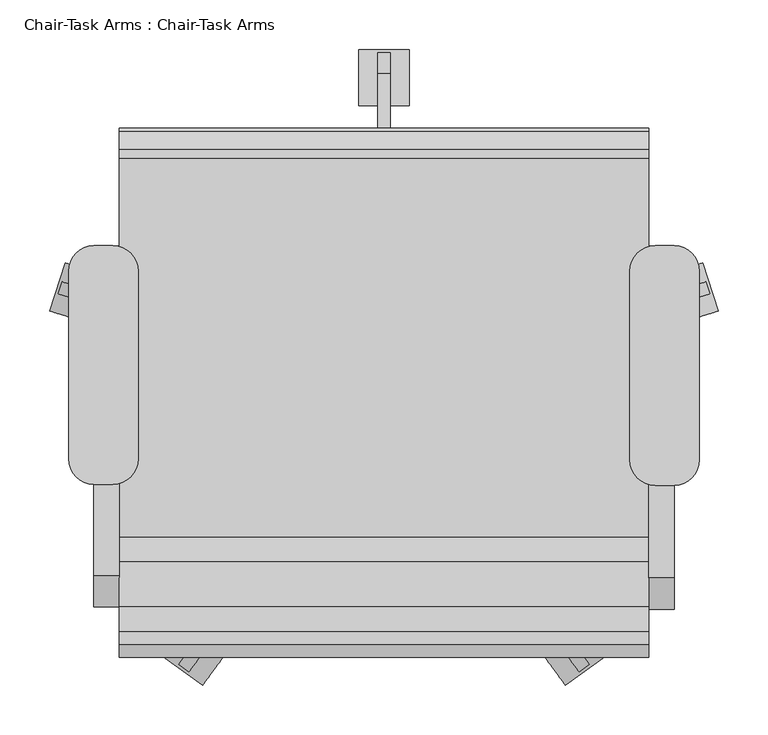
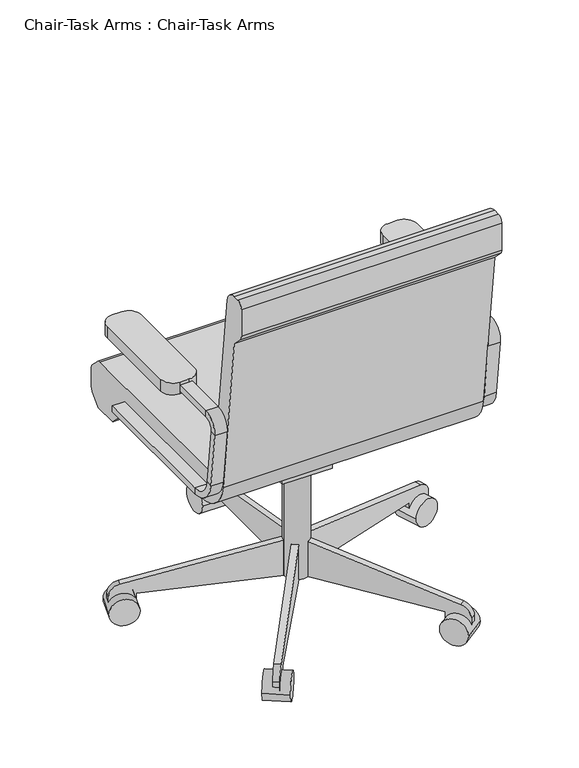
"""IFC4 building model written with IfcOpenShell, lengths in millimetres: furniture geometry, Chair-Task Arms : Chair-Task Arms."""

from ifc_helpers import new_model, si_unit, point, frame, frame_2d, origin, place, context, project, spatial, polyline, circle_curve, trimmed, segment, composite_curve, outline, extrude, source, transform, mapped, element, save
from ifc_brep_helpers import plane_surface, cylinder_surface, revolved_surface, advanced_brep


def chair_task_arms_chair_task_arms_fa5a08ef(model_context):
    return source(origin(), model_context, "Body", "SolidModel", [
        extrude(outline(composite_curve([segment(polyline([(433.0908197, -74.2028048), (414.0408197, -74.2028048)]), True, "CONTINUOUS"), segment(trimmed(circle_curve(frame_2d((414.0408197, -48.8028048)), 25.4), [point((414.0408197, -74.2028048))], [point((388.6408197, -48.8028048))], False, "CARTESIAN"), True, "CONTINUOUS"), segment(polyline([(388.6408197, -48.8028048), (388.6408197, 141.6319091)]), True, "CONTINUOUS"), segment(trimmed(circle_curve(frame_2d((414.0408197, 141.6319091)), 25.4), [point((388.6408197, 141.6319091))], [point((414.0408197, 167.0319091))], False, "CARTESIAN"), True, "CONTINUOUS"), segment(polyline([(414.0408197, 167.0319091), (433.0908197, 167.0319091)]), True, "CONTINUOUS"), segment(trimmed(circle_curve(frame_2d((433.0908197, 141.6319091)), 25.4), [point((433.0908197, 167.0319091))], [point((458.4908197, 141.6319091))], False, "CARTESIAN"), True, "CONTINUOUS"), segment(polyline([(458.4908197, 141.6319091), (458.4908197, -48.8028048)]), True, "CONTINUOUS"), segment(trimmed(circle_curve(frame_2d((433.0908197, -48.8028048)), 25.4), [point((458.4908197, -48.8028048))], [point((433.0908197, -74.2028048))], False, "CARTESIAN"), True, "CONTINUOUS")], self_intersect=False)), frame((0.0, 0.0, 596.9), z_axis=(0.0, 0.0, 1.0), x_axis=(1.0, 0.0, 0.0)), (0.0, 0.0, 1.0), 25.4),
        extrude(outline(composite_curve([segment(polyline([(-132.0591803, -73.1575984), (-151.1091803, -73.1575984)]), True, "CONTINUOUS"), segment(trimmed(circle_curve(frame_2d((-151.1091803, -47.7575984)), 25.4), [point((-151.1091803, -73.1575984))], [point((-176.5091803, -47.7575984))], False, "CARTESIAN"), True, "CONTINUOUS"), segment(polyline([(-176.5091803, -47.7575984), (-176.5091803, 141.6319091)]), True, "CONTINUOUS"), segment(trimmed(circle_curve(frame_2d((-151.1091803, 141.6319091)), 25.4), [point((-176.5091803, 141.6319091))], [point((-151.1091803, 167.0319091))], False, "CARTESIAN"), True, "CONTINUOUS"), segment(polyline([(-151.1091803, 167.0319091), (-132.0591803, 167.0319091)]), True, "CONTINUOUS"), segment(trimmed(circle_curve(frame_2d((-132.0591803, 141.6319091)), 25.4), [point((-132.0591803, 167.0319091))], [point((-106.6591803, 141.6319091))], False, "CARTESIAN"), True, "CONTINUOUS"), segment(polyline([(-106.6591803, 141.6319091), (-106.6591803, -47.7575984)]), True, "CONTINUOUS"), segment(trimmed(circle_curve(frame_2d((-132.0591803, -47.7575984)), 25.4), [point((-106.6591803, -47.7575984))], [point((-132.0591803, -73.1575984))], False, "CARTESIAN"), True, "CONTINUOUS")], self_intersect=False)), frame((0.0, 0.0, 596.9), z_axis=(0.0, 0.0, 1.0), x_axis=(1.0, 0.0, 0.0)), (0.0, 0.0, 1.0), 25.4),
        advanced_brep(
        [(-151.1091803, 167.0319091, 412.75), (-151.1091803, 167.0319091, 425.45), (-125.7091803, 167.0319091, 425.45), (-125.7091803, 167.0319091, 412.75), (-151.1091803, -126.2388651, 412.75), (-151.1091803, -126.2388651, 425.45), (-125.7091803, -126.2388651, 425.45), (-125.7091803, -126.2388651, 412.75), (-151.1091803, -170.3844094, 464.7064065), (-151.1091803, -182.9974221, 463.2225227), (-125.7091803, -170.3844094, 464.7064065), (-125.7091803, -182.9974221, 463.2225227), (-151.1091803, -196.7936301, 580.4902904), (-151.1091803, -184.1806174, 581.9741742), (-125.7091803, -184.1806174, 581.9741742), (-125.7091803, -196.7936301, 580.4902904), (-151.1091803, -165.2610984, 603.25), (-151.1091803, -165.2610984, 615.95), (-125.7091803, -165.2610984, 603.25), (-125.7091803, -165.2610984, 615.95), (-151.1091803, 18.9459016, 615.95), (-125.7091803, 18.9459016, 615.95), (-125.7091803, 18.9459016, 603.25), (-151.1091803, 18.9459016, 603.25)],
        [
            (0, 1),
            (1, 2),
            (2, 3),
            (3, 0),
            (0, 4),
            (4, 5),
            (5, 1),
            (5, 6),
            (6, 2),
            (6, 7),
            (7, 3),
            (7, 4),
            (8, 5, circle_curve(frame((-151.1091803, -126.2388651, 469.9), z_axis=(1.0, 0.0, 0.0), x_axis=(0.0, 0.0, -1.0)), 44.45)),
            (4, 9, circle_curve(frame((-151.1091803, -126.2388651, 469.9), z_axis=(-1.0, 0.0, 0.0), x_axis=(0.0, 0.0, -1.0)), 57.15)),
            (9, 8),
            (10, 6, circle_curve(frame((-125.7091803, -126.2388651, 469.9), z_axis=(1.0, 0.0, 0.0), x_axis=(0.0, 0.0, -1.0)), 44.45)),
            (8, 10),
            (11, 7, circle_curve(frame((-125.7091803, -126.2388651, 469.9), z_axis=(1.0, 0.0, 0.0), x_axis=(0.0, 0.0, -1.0)), 57.15)),
            (10, 11),
            (11, 9),
            (9, 12),
            (12, 13),
            (13, 8),
            (13, 14),
            (14, 10),
            (14, 15),
            (15, 11),
            (15, 12),
            (16, 13, circle_curve(frame((-151.1091803, -165.2610984, 584.2), z_axis=(1.0, 0.0, 0.0), x_axis=(0.0, -0.9931506043228768, -0.11684124756739202)), 19.05)),
            (12, 17, circle_curve(frame((-151.1091803, -165.2610984, 584.2), z_axis=(-1.0, 0.0, 0.0), x_axis=(0.0, -0.9931506043228768, -0.11684124756739202)), 31.75)),
            (17, 16),
            (18, 14, circle_curve(frame((-125.7091803, -165.2610984, 584.2), z_axis=(1.0, 0.0, 0.0), x_axis=(0.0, -0.9931506043228768, -0.11684124756739202)), 19.05)),
            (16, 18),
            (19, 15, circle_curve(frame((-125.7091803, -165.2610984, 584.2), z_axis=(1.0, 0.0, 0.0), x_axis=(0.0, -0.9931506043228768, -0.11684124756739202)), 31.75)),
            (18, 19),
            (19, 17),
            (20, 21),
            (21, 22),
            (22, 23),
            (23, 20),
            (17, 20),
            (23, 16),
            (22, 18),
            (21, 19),
        ],
        [
            plane_surface(frame((-152.608212, 167.0319091, 419.1), z_axis=(0.0, 1.0, 0.0), x_axis=(0.0, 0.0, -1.0))),
            plane_surface(frame((-151.1091803, 167.0319091, 412.75), z_axis=(-1.0, 0.0, 0.0), x_axis=(0.0, -1.0, 0.0))),
            plane_surface(frame((-151.1091803, 167.0319091, 425.45), z_axis=(0.0, 0.0, 1.0), x_axis=(0.0, -1.0, 0.0))),
            plane_surface(frame((-125.7091803, 167.0319091, 425.45), z_axis=(1.0, 0.0, 0.0), x_axis=(0.0, -1.0, 0.0))),
            plane_surface(frame((-125.7091803, 167.0319091, 412.75), z_axis=(0.0, 0.0, -1.0), x_axis=(0.0, -1.0, 0.0))),
            plane_surface(frame((-151.1091803, -126.2388651, 469.9), z_axis=(-1.0, 0.0, 0.0), x_axis=(0.0, 0.0, -1.0))),
            revolved_surface(polyline([(-151.1091803, -126.2388651, 425.45), (-125.7091803, -126.2388651, 425.45)]), (-138.4091803, -126.2388651, 469.9), (-1.0, 0.0, 0.0)),
            plane_surface(frame((-125.7091803, -126.2388651, 469.9), z_axis=(1.0, 0.0, 0.0), x_axis=(0.0, 0.0, -1.0))),
            cylinder_surface(frame((-138.4091803, -126.2388651, 469.9), z_axis=(-1.0, 0.0, 0.0), x_axis=(0.0, 0.0, -1.0)), 57.15),
            plane_surface(frame((-151.1091803, -182.9974221, 463.2225227), z_axis=(-1.0, 0.0, 0.0), x_axis=(0.0, -0.1168412475673856, 0.9931506043228776))),
            plane_surface(frame((-151.1091803, -170.3844094, 464.7064065), z_axis=(0.0, 0.9931506043228776, 0.1168412475673856), x_axis=(0.0, -0.1168412475673856, 0.9931506043228776))),
            plane_surface(frame((-125.7091803, -170.3844094, 464.7064065), z_axis=(1.0, 0.0, 0.0), x_axis=(0.0, -0.1168412475673856, 0.9931506043228776))),
            plane_surface(frame((-125.7091803, -182.9974221, 463.2225227), z_axis=(0.0, -0.9931506043228776, -0.1168412475673856), x_axis=(0.0, -0.1168412475673856, 0.9931506043228776))),
            plane_surface(frame((-151.1091803, -165.2610984, 584.2), z_axis=(-1.0, 0.0, 0.0), x_axis=(0.0, -0.9931506043228768, -0.11684124756739202))),
            revolved_surface(polyline([(-151.1091803, -184.1806174123508, 581.9741742338413), (-125.7091803, -184.1806174123508, 581.9741742338413)]), (-138.4091803, -165.2610984, 584.2), (-1.0, 0.0, 0.0)),
            plane_surface(frame((-125.7091803, -165.2610984, 584.2), z_axis=(1.0, 0.0, 0.0), x_axis=(0.0, -0.9931506043228768, -0.11684124756739202))),
            cylinder_surface(frame((-138.4091803, -165.2610984, 584.2), z_axis=(-1.0, 0.0, 0.0), x_axis=(0.0, -0.9931506043228768, -0.11684124756739202)), 31.75),
            plane_surface(frame((-152.608212, 18.9459016, 609.6), z_axis=(0.0, 1.0, 0.0), x_axis=(0.0, 0.0, 1.0))),
            plane_surface(frame((-151.1091803, -165.2610984, 615.95), z_axis=(-1.0, 0.0, 0.0), x_axis=(0.0, 1.0, 0.0))),
            plane_surface(frame((-151.1091803, -165.2610984, 603.25), z_axis=(0.0, 0.0, -1.0), x_axis=(0.0, 1.0, 0.0))),
            plane_surface(frame((-125.7091803, -165.2610984, 603.25), z_axis=(1.0, 0.0, 0.0), x_axis=(0.0, 1.0, 0.0))),
            plane_surface(frame((-125.7091803, -165.2610984, 615.95), z_axis=(0.0, 0.0, 1.0), x_axis=(0.0, 1.0, 0.0))),
        ],
        [
            (0, [[1, 2, 3, 4]]),
            (1, [[-1, 5, 6, 7]]),
            (2, [[-2, -7, 8, 9]]),
            (3, [[-3, -9, 10, 11]]),
            (4, [[-4, -11, 12, -5]]),
            (5, [[13, -6, 14, 15]]),
            (6, [[16, -8, -13, 17]]),
            (7, [[18, -10, -16, 19]]),
            (8, [[-14, -12, -18, 20]]),
            (9, [[-15, 21, 22, 23]]),
            (10, [[-17, -23, 24, 25]]),
            (11, [[-19, -25, 26, 27]]),
            (12, [[-20, -27, 28, -21]]),
            (13, [[29, -22, 30, 31]]),
            (14, [[32, -24, -29, 33]]),
            (15, [[34, -26, -32, 35]]),
            (16, [[-30, -28, -34, 36]]),
            (17, [[37, 38, 39, 40]]),
            (18, [[-31, 41, -40, 42]]),
            (19, [[-33, -42, -39, 43]]),
            (20, [[-35, -43, -38, 44]]),
            (21, [[-36, -44, -37, -41]]),
        ],
    ),
        advanced_brep(
        [(433.0908197, 167.0319091, 425.45), (433.0908197, 167.0319091, 412.75), (407.6908197, 167.0319091, 412.75), (407.6908197, 167.0319091, 425.45), (433.0908197, -128.329278, 425.45), (433.0908197, -128.329278, 412.75), (407.6908197, -128.329278, 412.75), (407.6908197, -128.329278, 425.45), (433.0908197, -185.0878351, 463.2225227), (433.0908197, -172.4748224, 464.7064065), (407.6908197, -185.0878351, 463.2225227), (407.6908197, -172.4748224, 464.7064065), (433.0908197, -186.2710303, 581.9741742), (433.0908197, -198.884043, 580.4902904), (407.6908197, -198.884043, 580.4902904), (407.6908197, -186.2710303, 581.9741742), (433.0908197, -167.3515113, 615.95), (433.0908197, -167.3515113, 603.25), (407.6908197, -167.3515113, 615.95), (407.6908197, -167.3515113, 603.25), (433.0908197, 18.9459016, 603.25), (407.6908197, 18.9459016, 603.25), (407.6908197, 18.9459016, 615.95), (433.0908197, 18.9459016, 615.95)],
        [
            (0, 1),
            (1, 2),
            (2, 3),
            (3, 0),
            (0, 4),
            (4, 5),
            (5, 1),
            (5, 6),
            (6, 2),
            (6, 7),
            (7, 3),
            (7, 4),
            (8, 5, circle_curve(frame((433.0908197, -128.329278, 469.9), z_axis=(1.0, 0.0, 0.0), x_axis=(0.0, 0.0, -1.0)), 57.15)),
            (4, 9, circle_curve(frame((433.0908197, -128.329278, 469.9), z_axis=(-1.0, 0.0, 0.0), x_axis=(0.0, 0.0, -1.0)), 44.45)),
            (9, 8),
            (10, 6, circle_curve(frame((407.6908197, -128.329278, 469.9), z_axis=(1.0, 0.0, 0.0), x_axis=(0.0, 0.0, -1.0)), 57.15)),
            (8, 10),
            (11, 7, circle_curve(frame((407.6908197, -128.329278, 469.9), z_axis=(1.0, 0.0, 0.0), x_axis=(0.0, 0.0, -1.0)), 44.45)),
            (10, 11),
            (11, 9),
            (9, 12),
            (12, 13),
            (13, 8),
            (13, 14),
            (14, 10),
            (14, 15),
            (15, 11),
            (15, 12),
            (16, 13, circle_curve(frame((433.0908197, -167.3515113, 584.2), z_axis=(1.0, 0.0, 0.0), x_axis=(0.0, -0.9931506043228767, -0.1168412475673929)), 31.75)),
            (12, 17, circle_curve(frame((433.0908197, -167.3515113, 584.2), z_axis=(-1.0, 0.0, 0.0), x_axis=(0.0, -0.9931506043228767, -0.1168412475673929)), 19.05)),
            (17, 16),
            (18, 14, circle_curve(frame((407.6908197, -167.3515113, 584.2), z_axis=(1.0, 0.0, 0.0), x_axis=(0.0, -0.9931506043228767, -0.1168412475673929)), 31.75)),
            (16, 18),
            (19, 15, circle_curve(frame((407.6908197, -167.3515113, 584.2), z_axis=(1.0, 0.0, 0.0), x_axis=(0.0, -0.9931506043228767, -0.1168412475673929)), 19.05)),
            (18, 19),
            (19, 17),
            (20, 21),
            (21, 22),
            (22, 23),
            (23, 20),
            (17, 20),
            (23, 16),
            (22, 18),
            (21, 19),
        ],
        [
            plane_surface(frame((406.191788, 167.0319091, 419.1), z_axis=(0.0, 1.0, 0.0), x_axis=(0.0, 0.0, -1.0))),
            plane_surface(frame((433.0908197, 167.0319091, 425.45), z_axis=(1.0, 0.0, 0.0), x_axis=(0.0, -1.0, 0.0))),
            plane_surface(frame((433.0908197, 167.0319091, 412.75), z_axis=(0.0, 0.0, -1.0), x_axis=(0.0, -1.0, 0.0))),
            plane_surface(frame((407.6908197, 167.0319091, 412.75), z_axis=(-1.0, 0.0, 0.0), x_axis=(0.0, -1.0, 0.0))),
            plane_surface(frame((407.6908197, 167.0319091, 425.45), z_axis=(0.0, 0.0, 1.0), x_axis=(0.0, -1.0, 0.0))),
            plane_surface(frame((433.0908197, -128.329278, 469.9), z_axis=(1.0, 0.0, 0.0), x_axis=(0.0, 0.0, -1.0))),
            cylinder_surface(frame((420.3908197, -128.329278, 469.9), z_axis=(-1.0, 0.0, 0.0), x_axis=(0.0, 0.0, -1.0)), 57.15),
            plane_surface(frame((407.6908197, -128.329278, 469.9), z_axis=(-1.0, 0.0, 0.0), x_axis=(0.0, 0.0, -1.0))),
            revolved_surface(polyline([(407.6908197, -128.329278, 425.45), (433.0908197, -128.329278, 425.45)]), (420.3908197, -128.329278, 469.9), (-1.0, 0.0, 0.0)),
            plane_surface(frame((433.0908197, -172.4748224, 464.7064065), z_axis=(1.0, 0.0, 0.0), x_axis=(0.0, -0.11684124756738626, 0.9931506043228775))),
            plane_surface(frame((433.0908197, -185.0878351, 463.2225227), z_axis=(0.0, -0.9931506043228775, -0.11684124756738655), x_axis=(0.0, -0.11684124756738655, 0.9931506043228775))),
            plane_surface(frame((407.6908197, -185.0878351, 463.2225227), z_axis=(-1.0, 0.0, 0.0), x_axis=(0.0, -0.11684124756738626, 0.9931506043228775))),
            plane_surface(frame((407.6908197, -172.4748224, 464.7064065), z_axis=(0.0, 0.9931506043228775, 0.11684124756738626), x_axis=(0.0, -0.11684124756738626, 0.9931506043228775))),
            plane_surface(frame((433.0908197, -167.3515113, 584.2), z_axis=(1.0, 0.0, 0.0), x_axis=(0.0, -0.9931506043228767, -0.1168412475673929))),
            cylinder_surface(frame((420.3908197, -167.3515113, 584.2), z_axis=(-1.0, 0.0, 0.0), x_axis=(0.0, -0.9931506043228767, -0.1168412475673929)), 31.75),
            plane_surface(frame((407.6908197, -167.3515113, 584.2), z_axis=(-1.0, 0.0, 0.0), x_axis=(0.0, -0.9931506043228767, -0.1168412475673929))),
            revolved_surface(polyline([(407.6908197, -186.2710303123508, 581.9741742338412), (433.0908197, -186.2710303123508, 581.9741742338412)]), (420.3908197, -167.3515113, 584.2), (-1.0, 0.0, 0.0)),
            plane_surface(frame((406.191788, 18.9459016, 609.6), z_axis=(0.0, 1.0, 0.0), x_axis=(0.0, 0.0, 1.0))),
            plane_surface(frame((433.0908197, -167.3515113, 603.25), z_axis=(1.0, 0.0, 0.0), x_axis=(0.0, 1.0, 0.0))),
            plane_surface(frame((433.0908197, -167.3515113, 615.95), z_axis=(0.0, 0.0, 1.0), x_axis=(0.0, 1.0, 0.0))),
            plane_surface(frame((407.6908197, -167.3515113, 615.95), z_axis=(-1.0, 0.0, 0.0), x_axis=(0.0, 1.0, 0.0))),
            plane_surface(frame((407.6908197, -167.3515113, 603.25), z_axis=(0.0, 0.0, -1.0), x_axis=(0.0, 1.0, 0.0))),
        ],
        [
            (0, [[1, 2, 3, 4]]),
            (1, [[-1, 5, 6, 7]]),
            (2, [[-2, -7, 8, 9]]),
            (3, [[-3, -9, 10, 11]]),
            (4, [[-4, -11, 12, -5]]),
            (5, [[13, -6, 14, 15]]),
            (6, [[16, -8, -13, 17]]),
            (7, [[18, -10, -16, 19]]),
            (8, [[-14, -12, -18, 20]]),
            (9, [[-15, 21, 22, 23]]),
            (10, [[-17, -23, 24, 25]]),
            (11, [[-19, -25, 26, 27]]),
            (12, [[-20, -27, 28, -21]]),
            (13, [[29, -22, 30, 31]]),
            (14, [[32, -24, -29, 33]]),
            (15, [[34, -26, -32, 35]]),
            (16, [[-30, -28, -34, 36]]),
            (17, [[37, 38, 39, 40]]),
            (18, [[-31, 41, -40, 42]]),
            (19, [[-33, -42, -39, 43]]),
            (20, [[-35, -43, -38, 44]]),
            (21, [[-36, -44, -37, -41]]),
        ],
    ),
        extrude(outline(composite_curve([segment(trimmed(circle_curve(frame_2d((140.9908197, 18.9459016)), 25.4), [point((115.5908197, 18.9459016))], [point((166.3908197, 18.9459016))], False, "CARTESIAN"), True, "CONTINUOUS"), segment(trimmed(circle_curve(frame_2d((140.9908197, 18.9459016)), 25.4), [point((166.3908197, 18.9459016))], [point((115.5908197, 18.9459016))], False, "CARTESIAN"), True, "CONTINUOUS")], self_intersect=False)), frame((0.0, 0.0, 53.5835944), z_axis=(0.0, 0.0, 1.0), x_axis=(1.0, 0.0, 0.0)), (0.0, 0.0, 1.0), 330.5914056),
        extrude(outline(composite_curve([segment(trimmed(circle_curve(frame_2d((0.0, -28.2002727)), 28.2002727), [point((0.0, -56.4005455))], [point((0.0, 0.0))], False, "CARTESIAN"), True, "CONTINUOUS"), segment(trimmed(circle_curve(frame_2d((0.0, -28.2002727)), 28.2002727), [point((0.0, 0.0))], [point((0.0, -56.4005455))], False, "CARTESIAN"), True, "CONTINUOUS")], self_intersect=False)), frame((477.6203484, 101.6163254, 28.1835944), z_axis=(-0.3090169943749423, 0.9510565162951553, 0.0), x_axis=(0.0, 0.0, 1.0)), (0.0, 0.0, 1.0), 50.8),
        extrude(outline(composite_curve([segment(polyline([(-25.4, 0.0), (0.0, 0.0), (0.0, -50.8), (-24.303053, -50.8)]), True, "CONTINUOUS"), segment(trimmed(circle_curve(frame_2d((-24.303053, -25.4)), 25.4), [point((-24.303053, -50.8))], [point((-49.3171699, -29.8106637))], False, "CARTESIAN"), True, "CONTINUOUS"), segment(polyline([(-49.3171699, -29.8106637), (-101.6, 266.7), (-101.6, 292.1), (-25.4, 292.1), (-25.4, 0.0)]), True, "CONTINUOUS")], self_intersect=False)), frame((420.756686, 103.1705568, 28.1835944), z_axis=(-0.3090169943749423, 0.9510565162951553, 0.0), x_axis=(0.0, 0.0, -1.0)), (0.0, 0.0, 1.0), 12.7),
        extrude(outline(composite_curve([segment(trimmed(circle_curve(frame_2d((0.0, -28.2002727)), 28.2002727), [point((0.0, -56.4005455))], [point((0.0, 0.0))], False, "CARTESIAN"), True, "CONTINUOUS"), segment(trimmed(circle_curve(frame_2d((0.0, -28.2002727)), 28.2002727), [point((0.0, 0.0))], [point((0.0, -56.4005455))], False, "CARTESIAN"), True, "CONTINUOUS")], self_intersect=False)), frame((323.63931, -275.6612394, 28.1835944), z_axis=(0.8090169943749499, 0.5877852522924699, 0.0), x_axis=(0.0, 0.0, 1.0)), (0.0, 0.0, 1.0), 50.8),
        extrude(outline(composite_curve([segment(polyline([(-25.4, 0.0), (0.0, 0.0), (0.0, -50.8), (-24.303053, -50.8)]), True, "CONTINUOUS"), segment(trimmed(circle_curve(frame_2d((-24.303053, -25.3999999)), 25.4), [point((-24.303053, -50.8))], [point((-49.3171699, -29.8106636))], False, "CARTESIAN"), True, "CONTINUOUS"), segment(polyline([(-49.3171699, -29.8106636), (-101.6, 266.7), (-101.6, 292.1), (-25.4, 292.1), (-25.4, 0.0)]), True, "CONTINUOUS")], self_intersect=False)), frame((307.545634, -221.1003988, 28.1835944), z_axis=(0.8090169943749499, 0.5877852522924699, 0.0), x_axis=(0.0, 0.0, -1.0)), (0.0, 0.0, 1.0), 12.7),
        extrude(outline(composite_curve([segment(trimmed(circle_curve(frame_2d((0.0, -28.2002727)), 28.2002727), [point((0.0, -56.4005455))], [point((0.0, 0.0))], False, "CARTESIAN"), True, "CONTINUOUS"), segment(trimmed(circle_curve(frame_2d((0.0, -28.2002727)), 28.2002727), [point((0.0, 0.0))], [point((0.0, -56.4005455))], False, "CARTESIAN"), True, "CONTINUOUS")], self_intersect=False)), frame((-41.6576707, -275.6612394, 28.1835944), z_axis=(-0.8090169943749458, 0.5877852522924754, 0.0), x_axis=(0.0, 0.0, -1.0)), (0.0, 0.0, 1.0), 50.8),
        extrude(outline(composite_curve([segment(polyline([(25.4, 0.0), (25.4, 292.1), (101.6, 292.1), (101.6, 266.7), (49.3171699, -29.8106637)]), True, "CONTINUOUS"), segment(trimmed(circle_curve(frame_2d((24.303053, -25.3999999)), 25.4), [point((49.3171699, -29.8106637))], [point((24.303053, -50.8))], False, "CARTESIAN"), True, "CONTINUOUS"), segment(polyline([(24.303053, -50.8), (0.0, -50.8), (0.0, 0.0), (25.4, 0.0)]), True, "CONTINUOUS")], self_intersect=False)), frame((-25.5639946, -221.1003988, 28.1835944), z_axis=(-0.8090169943749459, 0.5877852522924754, 0.0), x_axis=(0.0, 0.0, 1.0)), (0.0, 0.0, 1.0), 12.7),
        extrude(outline(composite_curve([segment(trimmed(circle_curve(frame_2d((0.0, -28.2002727)), 28.2002727), [point((0.0, -56.4005454))], [point((0.0, 0.0))], False, "CARTESIAN"), True, "CONTINUOUS"), segment(trimmed(circle_curve(frame_2d((0.0, -28.2002727)), 28.2002727), [point((0.0, 0.0))], [point((0.0, -56.4005454))], False, "CARTESIAN"), True, "CONTINUOUS")], self_intersect=False)), frame((-195.638709, 101.6163254, 28.1835944), z_axis=(0.3090169943749487, 0.9510565162951532, 0.0), x_axis=(0.0, 0.0, -1.0)), (0.0, 0.0, 1.0), 50.8),
        extrude(outline(composite_curve([segment(polyline([(25.4, 0.0), (25.4, 292.1000001), (101.6, 292.1000001), (101.6, 266.7), (49.3171699, -29.8106636)]), True, "CONTINUOUS"), segment(trimmed(circle_curve(frame_2d((24.303053, -25.4)), 25.4), [point((49.3171699, -29.8106636))], [point((24.303053, -50.8))], False, "CARTESIAN"), True, "CONTINUOUS"), segment(polyline([(24.303053, -50.8), (0.0, -50.8), (0.0, 0.0), (25.4, 0.0)]), True, "CONTINUOUS")], self_intersect=False)), frame((-138.7750467, 103.1705568, 28.1835944), z_axis=(0.3090169943749487, 0.9510565162951532, 0.0), x_axis=(0.0, 0.0, 1.0)), (0.0, 0.0, 1.0), 12.7),
        extrude(outline(composite_curve([segment(trimmed(circle_curve(frame_2d((336.4459016, 28.1835944)), 28.2002727), [point((308.2456289, 28.1835944))], [point((364.6461744, 28.1835944))], False, "CARTESIAN"), True, "CONTINUOUS"), segment(trimmed(circle_curve(frame_2d((336.4459016, 28.1835944)), 28.2002727), [point((364.6461744, 28.1835944))], [point((308.2456289, 28.1835944))], False, "CARTESIAN"), True, "CONTINUOUS")], self_intersect=False)), frame((115.5908197, 0.0, 0.0), z_axis=(1.0, 0.0, 0.0), x_axis=(0.0, 1.0, 0.0)), (0.0, 0.0, 1.0), 50.8),
        extrude(outline(composite_curve([segment(polyline([(311.0459016, 53.5835944), (18.9459016, 53.5835944), (18.9459016, 129.7835944), (44.3459016, 129.7835944), (340.8565654, 77.5007643)]), True, "CONTINUOUS"), segment(trimmed(circle_curve(frame_2d((336.4459016, 52.4866474)), 25.4), [point((340.8565654, 77.5007643))], [point((361.8459016, 52.4866474))], False, "CARTESIAN"), True, "CONTINUOUS"), segment(polyline([(361.8459016, 52.4866474), (361.8459016, 28.1835944), (311.0459016, 28.1835944), (311.0459016, 53.5835944)]), True, "CONTINUOUS")], self_intersect=False)), frame((134.6408197, 0.0, 0.0), z_axis=(1.0, 0.0, 0.0), x_axis=(0.0, 1.0, 0.0)), (0.0, 0.0, 1.0), 12.7),
        extrude(outline(polyline([(69.7459016, 383.7835944), (69.7459016, 371.0835944), (18.9459016, 283.0954134), (-19.1540984, 283.0954134), (-19.1540984, 383.7835944), (69.7459016, 383.7835944)])), frame((90.1908197, 0.0, 0.0), z_axis=(1.0, 0.0, 0.0), x_axis=(0.0, 1.0, 0.0)), (0.0, 0.0, 1.0), 101.6),
        extrude(outline(composite_curve([segment(polyline([(-126.2050455, 457.2), (255.0102301, 457.2)]), True, "CONTINUOUS"), segment(trimmed(circle_curve(frame_2d((255.0102301, 444.5)), 12.7), [point((255.0102301, 457.2))], [point((263.9604301, 453.510212))], False, "CARTESIAN"), True, "CONTINUOUS"), segment(polyline([(263.9604301, 453.510212), (281.8961016, 435.6939999)]), True, "CONTINUOUS"), segment(trimmed(circle_curve(frame_2d((272.9459016, 426.6837879)), 12.7), [point((281.8961016, 435.6939999))], [point((285.6459016, 426.6837879))], False, "CARTESIAN"), True, "CONTINUOUS"), segment(polyline([(285.6459016, 426.6837879), (285.6459016, 391.6405184)]), True, "CONTINUOUS"), segment(trimmed(circle_curve(frame_2d((260.2459016, 391.6405184)), 25.4), [point((285.6459016, 391.6405184))], [point((278.2663256, 373.7401184))], False, "CARTESIAN"), True, "CONTINUOUS"), segment(polyline([(278.2663256, 373.7401184), (260.2470284, 355.6), (209.4470284, 355.6), (181.0744602, 383.7835944), (-107.1089978, 383.7835944)]), True, "CONTINUOUS"), segment(trimmed(circle_curve(frame_2d((-107.1089978, 459.9835944)), 76.2), [point((-107.1089978, 383.7835944))], [point((-182.7870738, 451.0802913))], False, "CARTESIAN"), True, "CONTINUOUS"), segment(polyline([(-182.7870738, 451.0802913), (-222.3540984, 787.4), (-244.0343545, 809.0802561)]), True, "CONTINUOUS"), segment(trimmed(circle_curve(frame_2d((-235.0540984, 818.0605122)), 12.7), [point((-244.0343545, 809.0802561))], [point((-247.7540984, 818.0605122))], False, "CARTESIAN"), True, "CONTINUOUS"), segment(polyline([(-247.7540984, 818.0605122), (-247.7540984, 876.3)]), True, "CONTINUOUS"), segment(trimmed(circle_curve(frame_2d((-235.0540984, 876.3)), 12.7), [point((-247.7540984, 876.3))], [point((-235.0540984, 889.0))], False, "CARTESIAN"), True, "CONTINUOUS"), segment(polyline([(-235.0540984, 889.0), (-222.1789239, 889.0)]), True, "CONTINUOUS"), segment(trimmed(circle_curve(frame_2d((-222.1789239, 863.6)), 25.4), [point((-222.1789239, 889.0))], [point((-196.9528985, 866.5677677))], False, "CARTESIAN"), True, "CONTINUOUS"), segment(polyline([(-196.9528985, 866.5677677), (-151.4310708, 479.6322323)]), True, "CONTINUOUS"), segment(trimmed(circle_curve(frame_2d((-126.2050455, 482.6)), 25.4), [point((-151.4310708, 479.6322323))], [point((-126.2050455, 457.2))], True, "CARTESIAN"), True, "CONTINUOUS")], self_intersect=False)), frame((-125.7091803, 0.0, 0.0), z_axis=(1.0, 0.0, 0.0), x_axis=(0.0, 1.0, 0.0)), (0.0, 0.0, 1.0), 533.4),
    ])


if __name__ == "__main__":
    model = new_model("IFC4")
    model_context = context("Model", 3, world=origin())
    ifc_project = project(units=[si_unit("LENGTHUNIT", "METRE", prefix="MILLI")], contexts=[model_context])
    site = spatial("IfcSite", under=ifc_project)
    building = spatial("IfcBuilding", under=site)
    placement = place(None, origin())
    chair_task_arms_chair_task_arms_shape = chair_task_arms_chair_task_arms_fa5a08ef(model_context)
    element("IfcFurniture", 1, ObjectType="Chair-Task Arms : Chair-Task Arms", at=placement, inside=building, context=model_context, shape_type="MappedRepresentation", body=[
        mapped(chair_task_arms_chair_task_arms_shape, transform((0.0, 0.0, 0.0), x_axis=(1.0, 0.0, 0.0), y_axis=(0.0, 1.0, 0.0), z_axis=(0.0, 0.0, 1.0))),
    ])
    save(model, "model.ifc")

# Revit data of these elements
# Type "Chair-Task Arms : Chair-Task Arms"
#   Assembly Code = "E2020200"
#   Base Material = Plastic, Opaque Black
#   Caster Material = Plastic, Opaque Black
#   Seat/Back Material = Textile - Slate Blue
# Element 1 (IfcFurniture, "Chair-Task Arms : Chair-Task Arms")
#   Materials on its faces: "Plastic, Opaque Black", "Textile - Slate Blue"
# Materials
#   "Plastic, Opaque Black": class "Plastic", colour RGB 0 0 0, transparency 0.7, Description = "Plastic, generic, opaque black", Cost = 0
#   "Textile - Slate Blue": class "Fabric", colour RGB 98 102 118, transparency 0
